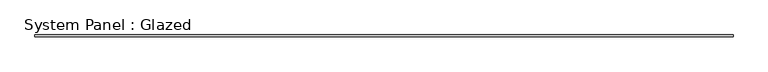
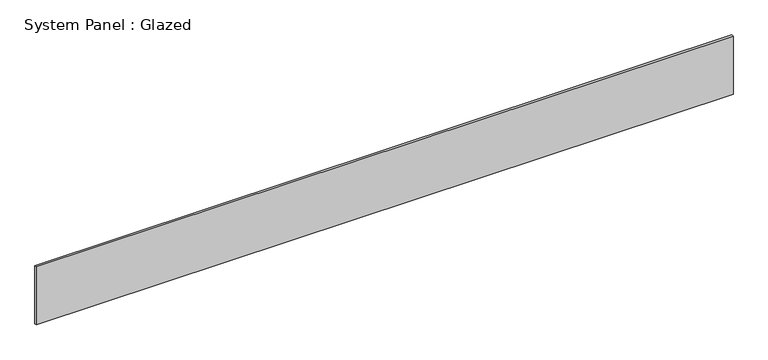
"""IFC4 building model written with IfcOpenShell, lengths in millimetres: plate geometry, System Panel : Glazed."""

from ifc_helpers import new_model, si_unit, origin, origin_with_axes, place, context, project, spatial, polyline, outline, extrude, source, transform, mapped, element, save


def system_panel_glazed_4881c73b(model_context):
    return source(origin(), model_context, "Body", "SweptSolid", [
        extrude(outline(polyline([(4184.65, 24.5), (-4184.65, 24.5), (-4184.65, 49.5), (4184.65, 49.5), (4184.65, 24.5)])), origin_with_axes(), (0.0, 0.0, 1.0), 737.3398437),
    ])


if __name__ == "__main__":
    model = new_model("IFC4")
    model_context = context("Model", 3, world=origin())
    ifc_project = project(units=[si_unit("LENGTHUNIT", "METRE", prefix="MILLI")], contexts=[model_context])
    site = spatial("IfcSite", under=ifc_project)
    building = spatial("IfcBuilding", under=site)
    placement = place(None, origin())
    system_panel_glazed_shape = system_panel_glazed_4881c73b(model_context)
    element("IfcPlate", 1, ObjectType="System Panel : Glazed", at=placement, inside=building, context=model_context, shape_type="MappedRepresentation", body=[
        mapped(system_panel_glazed_shape, transform((0.0, 0.0, 0.0), x_axis=(1.0, 0.0, 0.0), y_axis=(0.0, 1.0, 0.0), z_axis=(0.0, 0.0, 1.0))),
    ])
    save(model, "model.ifc")

# Revit data of these elements
# Type "System Panel : Glazed"
#   Keynote = "H11"
#   Construction Type Id = "GSP4R"
#   Analytic Construction = "1/8 in Pilkington single glazing"
#   Visual Light Transmittance = 0.9
#   Solar Heat Gain Coefficient = 0.86
#   Heat Transfer Coefficient (U) = 6.7069 W/(m²·K)
#   Define Thermal Properties by = 1
# Element 1 (IfcPlate, "System Panel : Glazed")
#   Materials on its faces: "Glass"
# Materials
#   "Glass": class "Glass", colour RGB 0 128 192, transparency 0.9, Description = "Soda Lime Glass", Cost = 0
